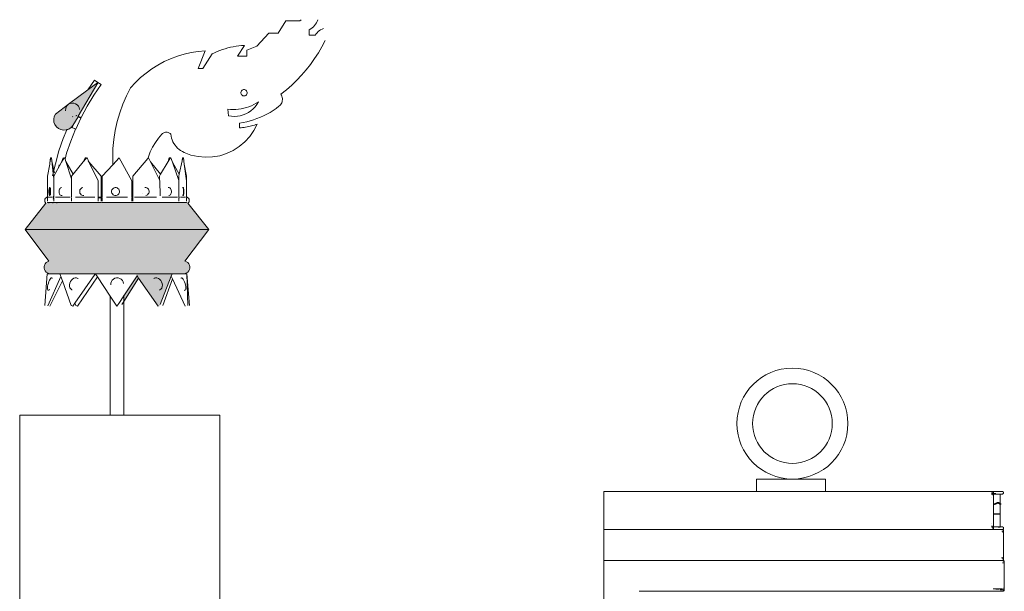
# Model space of a CAD drawing. Units: millimetres. Extents: x 2322 to 2394, y 1600 to 1790.
# Tile 5 of 5: x 2322 to 2380, y 1757 to 1790. Entities that reach past the tile are written whole.
import ezdxf

# ---------------------------------------------------------------- set-up
doc = ezdxf.new("R2010")
doc.units = ezdxf.units.MM
doc.layers.add('A-FURN-ACCS', color=8, linetype='Continuous', lineweight=18)
doc.layers.add('A-FURN-PATT', color=18, linetype='Continuous', lineweight=13)

msp = doc.modelspace()

# ---------------------------------------------------------------- hatches: boundary and pattern name
at = {"layer": 'A-FURN-PATT'}
h = msp.add_hatch(color=256, dxfattribs=at)
h.dxf.hatch_style = 1
h.paths.add_polyline_path([(2326.67, 1786.535), (2326.67, 1786.566), (2326.085, 1786.128), (2324.955, 1785.277), (2324.18, 1784.703), (2324.111, 1784.565), (2324.082, 1784.414), (2324.082, 1784.383), (2324.093, 1784.23), (2324.146, 1784.085), (2324.235, 1783.958), (2324.355, 1783.858), (2324.499, 1783.791), (2324.655, 1783.762), (2324.813, 1783.774), (2324.846, 1783.785), (2324.963, 1783.824), (2325.095, 1783.911), (2325.116, 1783.935), (2325.199, 1784.027), (2325.505, 1784.55), (2325.522, 1784.578)])
h = msp.add_hatch(color=256, dxfattribs=at)
h.dxf.hatch_style = 1
h.paths.add_polyline_path([(2331.932, 1779.508), (2331.431, 1779.508), (2328.723, 1779.508), (2328.671, 1779.508), (2326.915, 1779.508), (2326.693, 1779.508), (2325.129, 1779.508), (2324.26, 1779.508), (2324.078, 1779.508), (2323.654, 1779.508), (2322.407, 1777.93), (2333.179, 1777.93)])
h.paths.add_polyline_path([(2329.065, 1775.075), (2328.192, 1773.709), (2328.192, 1774.037), (2328.972, 1775.209), (2328.887, 1775.333), (2328.806, 1775.334), (2326.559, 1775.334), (2326.559, 1775.291), (2326.583, 1775.254), (2326.403, 1775.334), (2324.439, 1775.334), (2324.444, 1775.321), (2324.403, 1775.334), (2323.879, 1775.334), (2323.714, 1775.334), (2323.509, 1775.569), (2323.513, 1775.85), (2323.761, 1776.118), (2322.407, 1777.93), (2333.179, 1777.93), (2331.799, 1776.084), (2332.026, 1775.934), (2332.098, 1775.662), (2331.897, 1775.269), (2331.896, 1775.318), (2331.894, 1775.332), (2331.707, 1775.334), (2331.079, 1775.334), (2331.03, 1775.32), (2330.978, 1775.187), (2330.253, 1773.35)])
h.paths.add_polyline_path([(2330.421, 1774.493), (2330.451, 1774.574), (2330.46, 1774.664), (2330.448, 1774.759), (2330.415, 1774.851), (2330.364, 1774.935), (2330.298, 1775.004), (2330.222, 1775.053), (2330.104, 1775.093), (2330.07, 1775.083), (2330.227, 1775.078), (2330.435, 1774.861), (2330.473, 1774.563)], flags=16)

# ---------------------------------------------------------------- linework, layer by layer
at = {"layer": 'A-FURN-ACCS'}
for p, q in [((2337.261, 1789.455), (2337.707, 1790.174)), ((2337.707, 1790.174), (2338.529, 1790.174)), ((2338.529, 1790.174), (2338.606, 1790.244)), ((2339.456, 1789.973), (2339.394, 1789.895)), ((2339.51, 1790.056), (2339.456, 1789.973)), ((2339.556, 1790.144), (2339.51, 1790.056)), ((2339.593, 1790.236), (2339.556, 1790.144)), ((2336.01, 1788.693), (2336.709, 1789.455)), ((2336.709, 1789.455), (2337.261, 1789.455)), ((2339.17, 1789.701), (2339.084, 1789.652)), ((2339.084, 1789.652), (2339.084, 1789.334)), ((2339.251, 1789.758), (2339.17, 1789.701)), ((2339.326, 1789.823), (2339.251, 1789.758)), ((2339.394, 1789.895), (2339.326, 1789.823)), ((2339.436, 1789.334), (2339.487, 1789.409)), ((2339.487, 1789.409), (2339.544, 1789.479)), ((2339.544, 1789.479), (2339.608, 1789.542)), ((2339.608, 1789.542), (2339.677, 1789.6)), ((2339.677, 1789.6), (2339.752, 1789.65)), ((2339.752, 1789.65), (2339.832, 1789.693)), ((2339.832, 1789.693), (2339.915, 1789.727)), ((2339.084, 1789.334), (2339.436, 1789.334)), ((2340.022, 1789.023), (2339.828, 1788.659)), ((2331.738, 1788.218), (2332.147, 1788.31)), ((2332.147, 1788.31), (2332.561, 1788.373)), ((2332.561, 1788.373), (2332.978, 1788.408)), ((2332.978, 1788.408), (2332.568, 1787.37)), ((2332.827, 1787.37), (2333.378, 1788.231)), ((2333.378, 1788.231), (2333.526, 1788.304)), ((2333.526, 1788.304), (2333.677, 1788.371)), ((2333.677, 1788.371), (2333.829, 1788.433)), ((2333.829, 1788.433), (2333.984, 1788.489)), ((2333.984, 1788.489), (2334.141, 1788.54)), ((2334.141, 1788.54), (2334.299, 1788.585)), ((2334.299, 1788.585), (2334.459, 1788.624)), ((2334.459, 1788.624), (2334.621, 1788.658)), ((2334.621, 1788.658), (2334.783, 1788.686)), ((2334.783, 1788.686), (2334.946, 1788.708)), ((2335.275, 1788.734), (2334.869, 1788.101)), ((2334.946, 1788.708), (2335.11, 1788.724)), ((2335.11, 1788.724), (2335.275, 1788.734)), ((2335.41, 1788.454), (2336.01, 1788.693)), ((2335.41, 1788.101), (2335.41, 1788.454)), ((2339.619, 1788.304), (2339.394, 1787.958)), ((2339.828, 1788.659), (2339.619, 1788.304)), ((2330.193, 1787.583), (2330.562, 1787.78)), ((2330.562, 1787.78), (2330.944, 1787.953)), ((2330.944, 1787.953), (2331.337, 1788.099)), ((2331.337, 1788.099), (2331.738, 1788.218)), ((2334.869, 1788.101), (2335.41, 1788.101)), ((2339.394, 1787.958), (2339.154, 1787.623)), ((2329.178, 1786.845), (2329.5, 1787.114)), ((2329.5, 1787.114), (2329.839, 1787.36)), ((2329.839, 1787.36), (2330.193, 1787.583)), ((2332.568, 1787.37), (2332.827, 1787.37)), ((2338.899, 1787.299), (2338.63, 1786.987)), ((2339.154, 1787.623), (2338.899, 1787.299)), ((2326.67, 1786.535), (2325.522, 1784.578)), ((2326.476, 1786.699), (2326.085, 1786.128)), ((2326.67, 1786.566), (2326.085, 1786.128)), ((2326.67, 1786.566), (2326.476, 1786.699)), ((2326.67, 1786.535), (2326.67, 1786.566)), ((2326.864, 1786.433), (2326.67, 1786.566)), ((2328.594, 1786.246), (2328.876, 1786.556)), ((2328.876, 1786.556), (2329.178, 1786.845)), ((2338.347, 1786.687), (2338.051, 1786.4)), ((2338.63, 1786.987), (2338.347, 1786.687)), ((2326.085, 1786.128), (2324.955, 1785.277)), ((2326.434, 1785.805), (2326.864, 1786.433)), ((2328.594, 1786.246), (2328.353, 1785.77)), ((2335.066, 1785.929), (2335.067, 1785.979)), ((2335.079, 1785.882), (2335.066, 1785.929)), ((2335.067, 1785.979), (2335.08, 1786.026)), ((2335.08, 1786.026), (2335.104, 1786.068)), ((2335.104, 1786.068), (2335.139, 1786.103)), ((2335.139, 1786.103), (2335.182, 1786.127)), ((2335.182, 1786.127), (2335.229, 1786.14)), ((2335.229, 1786.14), (2335.278, 1786.139)), ((2335.278, 1786.139), (2335.326, 1786.126)), ((2335.326, 1786.126), (2335.368, 1786.102)), ((2335.368, 1786.102), (2335.403, 1786.067)), ((2335.403, 1786.067), (2335.427, 1786.024)), ((2335.439, 1785.928), (2335.426, 1785.88)), ((2335.427, 1786.024), (2335.439, 1785.977)), ((2335.439, 1785.977), (2335.439, 1785.928)), ((2337.743, 1786.126), (2337.422, 1785.867)), ((2338.051, 1786.4), (2337.743, 1786.126)), ((2325.051, 1785.324), (2325.156, 1785.346)), ((2325.156, 1785.346), (2325.263, 1785.341)), ((2325.263, 1785.341), (2325.365, 1785.308)), ((2326.042, 1785.161), (2326.434, 1785.805)), ((2328.353, 1785.77), (2328.142, 1785.279)), ((2335.103, 1785.839), (2335.079, 1785.882)), ((2335.138, 1785.804), (2335.103, 1785.839)), ((2335.18, 1785.78), (2335.138, 1785.804)), ((2335.227, 1785.767), (2335.18, 1785.78)), ((2335.276, 1785.767), (2335.227, 1785.767)), ((2335.324, 1785.779), (2335.276, 1785.767)), ((2335.367, 1785.803), (2335.324, 1785.779)), ((2335.401, 1785.838), (2335.367, 1785.803)), ((2335.426, 1785.88), (2335.401, 1785.838)), ((2335.966, 1785.337), (2335.828, 1785.261)), ((2336.099, 1785.421), (2335.966, 1785.337)), ((2336.099, 1785.421), (2336.008, 1785.273)), ((2337.422, 1785.867), (2337.455, 1785.81)), ((2337.465, 1785.364), (2337.435, 1785.306)), ((2337.455, 1785.81), (2337.48, 1785.749)), ((2337.488, 1785.426), (2337.465, 1785.364)), ((2337.48, 1785.749), (2337.498, 1785.686)), ((2337.502, 1785.49), (2337.488, 1785.426)), ((2337.498, 1785.686), (2337.508, 1785.621)), ((2337.509, 1785.555), (2337.502, 1785.49)), ((2337.508, 1785.621), (2337.509, 1785.555)), ((2324.955, 1785.277), (2324.18, 1784.703)), ((2324.778, 1784.919), (2324.784, 1785.022)), ((2324.779, 1784.915), (2324.778, 1784.919)), ((2324.778, 1784.901), (2324.779, 1784.915)), ((2324.784, 1785.022), (2324.817, 1785.121)), ((2324.817, 1785.121), (2324.875, 1785.208)), ((2324.875, 1785.208), (2324.955, 1785.277)), ((2324.955, 1785.277), (2325.051, 1785.324)), ((2325.365, 1785.308), (2325.455, 1785.252)), ((2325.455, 1785.252), (2325.527, 1785.175)), ((2325.527, 1785.175), (2325.576, 1785.082)), ((2325.576, 1785.082), (2325.598, 1784.981)), ((2325.597, 1784.966), (2325.598, 1784.981)), ((2325.597, 1784.966), (2325.598, 1784.963)), ((2326.042, 1785.161), (2325.685, 1784.496)), ((2327.961, 1784.776), (2327.812, 1784.264)), ((2328.142, 1785.279), (2327.961, 1784.776)), ((2334.462, 1784.972), (2334.306, 1784.985)), ((2334.306, 1784.985), (2334.344, 1784.595)), ((2334.619, 1784.968), (2334.462, 1784.972)), ((2334.776, 1784.973), (2334.619, 1784.968)), ((2334.932, 1784.987), (2334.776, 1784.973)), ((2335.087, 1785.011), (2334.932, 1784.987)), ((2335.241, 1785.043), (2335.087, 1785.011)), ((2335.392, 1785.085), (2335.241, 1785.043)), ((2335.509, 1784.802), (2335.357, 1784.721)), ((2335.541, 1785.135), (2335.392, 1785.085)), ((2335.652, 1784.9), (2335.509, 1784.802)), ((2335.687, 1785.194), (2335.541, 1785.135)), ((2335.783, 1785.012), (2335.652, 1784.9)), ((2335.828, 1785.261), (2335.687, 1785.194)), ((2335.903, 1785.137), (2335.783, 1785.012)), ((2336.008, 1785.273), (2335.903, 1785.137)), ((2336.778, 1784.805), (2336.593, 1784.702)), ((2336.958, 1784.916), (2336.778, 1784.805)), ((2337.134, 1785.034), (2336.958, 1784.916)), ((2337.304, 1785.16), (2337.134, 1785.034)), ((2337.354, 1785.203), (2337.304, 1785.16)), ((2337.397, 1785.252), (2337.354, 1785.203)), ((2337.435, 1785.306), (2337.397, 1785.252)), ((2324.111, 1784.565), (2324.082, 1784.414)), ((2324.082, 1784.383), (2324.082, 1784.414)), ((2324.082, 1784.383), (2324.093, 1784.23)), ((2324.093, 1784.23), (2324.146, 1784.085)), ((2324.18, 1784.703), (2324.111, 1784.565)), ((2325.194, 1784.555), (2325.185, 1784.537)), ((2325.505, 1784.55), (2325.199, 1784.027)), ((2325.367, 1783.817), (2325.673, 1784.471)), ((2325.386, 1784.605), (2325.405, 1784.597)), ((2325.438, 1784.619), (2325.425, 1784.626)), ((2325.522, 1784.578), (2325.505, 1784.55)), ((2325.673, 1784.471), (2325.505, 1784.55)), ((2325.522, 1784.578), (2325.685, 1784.496)), ((2327.812, 1784.264), (2327.695, 1783.743)), ((2334.515, 1784.571), (2334.344, 1784.595)), ((2334.688, 1784.565), (2334.515, 1784.571)), ((2334.86, 1784.577), (2334.688, 1784.565)), ((2335.031, 1784.607), (2334.86, 1784.577)), ((2335.201, 1784.208), (2334.992, 1784.171)), ((2335.197, 1784.656), (2335.031, 1784.607)), ((2335.357, 1784.721), (2335.197, 1784.656)), ((2335.408, 1784.253), (2335.201, 1784.208)), ((2335.612, 1784.307), (2335.408, 1784.253)), ((2335.815, 1784.369), (2335.612, 1784.307)), ((2336.014, 1784.44), (2335.815, 1784.369)), ((2336.211, 1784.519), (2336.014, 1784.44)), ((2336.404, 1784.606), (2336.211, 1784.519)), ((2336.593, 1784.702), (2336.404, 1784.606)), ((2324.146, 1784.085), (2324.235, 1783.958)), ((2324.235, 1783.958), (2324.355, 1783.858)), ((2324.355, 1783.858), (2324.499, 1783.791)), ((2324.499, 1783.791), (2324.655, 1783.762)), ((2324.846, 1783.785), (2324.641, 1783.277)), ((2324.655, 1783.762), (2324.813, 1783.774)), ((2324.813, 1783.774), (2324.846, 1783.785)), ((2324.846, 1783.785), (2324.963, 1783.824)), ((2324.861, 1783.82), (2324.846, 1783.785)), ((2324.963, 1783.824), (2325.095, 1783.911)), ((2325.082, 1783.113), (2325.364, 1783.812)), ((2325.085, 1783.934), (2325.107, 1783.925)), ((2325.095, 1783.911), (2325.107, 1783.925)), ((2325.116, 1783.935), (2325.099, 1783.943)), ((2325.107, 1783.925), (2325.116, 1783.935)), ((2325.107, 1783.925), (2325.364, 1783.812)), ((2325.116, 1783.935), (2325.199, 1784.027)), ((2325.116, 1783.935), (2325.367, 1783.817)), ((2325.154, 1783.917), (2325.149, 1783.906)), ((2325.232, 1784.084), (2325.154, 1783.917)), ((2327.695, 1783.743), (2327.611, 1783.215)), ((2330.546, 1783.61), (2330.502, 1783.587)), ((2330.593, 1783.627), (2330.546, 1783.61)), ((2330.641, 1783.637), (2330.593, 1783.627)), ((2330.691, 1783.641), (2330.641, 1783.637)), ((2330.74, 1783.637), (2330.691, 1783.641)), ((2330.789, 1783.627), (2330.74, 1783.637)), ((2330.835, 1783.61), (2330.789, 1783.627)), ((2330.879, 1783.587), (2330.835, 1783.61)), ((2334.992, 1784.171), (2334.992, 1783.901)), ((2334.992, 1783.901), (2335.081, 1783.905)), ((2335.081, 1783.905), (2335.169, 1783.912)), ((2335.169, 1783.912), (2335.257, 1783.921)), ((2335.257, 1783.921), (2335.345, 1783.933)), ((2335.345, 1783.933), (2335.432, 1783.948)), ((2335.432, 1783.948), (2335.519, 1783.965)), ((2335.519, 1783.965), (2335.605, 1783.984)), ((2335.832, 1783.74), (2335.589, 1783.389)), ((2335.605, 1783.984), (2335.691, 1784.007)), ((2335.691, 1784.007), (2335.776, 1784.031)), ((2335.776, 1784.031), (2335.861, 1784.059)), ((2336.027, 1784.12), (2335.832, 1783.74)), ((2335.861, 1784.059), (2335.944, 1784.088)), ((2335.944, 1784.088), (2336.027, 1784.12)), ((2324.641, 1783.277), (2324.388, 1782.539)), ((2324.837, 1782.399), (2325.082, 1783.113)), ((2327.611, 1783.215), (2327.559, 1782.684)), ((2330.048, 1783.031), (2329.888, 1782.763)), ((2330.227, 1783.284), (2330.048, 1783.031)), ((2330.426, 1783.523), (2330.227, 1783.284)), ((2330.462, 1783.558), (2330.426, 1783.523)), ((2330.502, 1783.587), (2330.462, 1783.558)), ((2330.919, 1783.558), (2330.879, 1783.587)), ((2330.955, 1783.523), (2330.919, 1783.558)), ((2330.972, 1783.409), (2330.955, 1783.523)), ((2330.999, 1783.296), (2330.972, 1783.409)), ((2331.036, 1783.186), (2330.999, 1783.296)), ((2331.082, 1783.08), (2331.036, 1783.186)), ((2331.137, 1782.978), (2331.082, 1783.08)), ((2335.303, 1783.073), (2334.976, 1782.798)), ((2335.589, 1783.389), (2335.303, 1783.073)), ((2324.388, 1782.539), (2324.175, 1781.789)), ((2327.559, 1782.684), (2327.54, 1782.15)), ((2329.751, 1782.484), (2329.636, 1782.195)), ((2329.888, 1782.763), (2329.751, 1782.484)), ((2331.201, 1782.882), (2331.137, 1782.978)), ((2331.273, 1782.791), (2331.201, 1782.882)), ((2331.353, 1782.707), (2331.273, 1782.791)), ((2331.439, 1782.63), (2331.353, 1782.707)), ((2331.532, 1782.561), (2331.439, 1782.63)), ((2331.631, 1782.5), (2331.532, 1782.561)), ((2331.734, 1782.448), (2331.631, 1782.5)), ((2332.135, 1782.3), (2331.734, 1782.448)), ((2334.617, 1782.567), (2334.23, 1782.386)), ((2334.976, 1782.798), (2334.617, 1782.567)), ((2323.85, 1781.835), (2323.888, 1782.128)), ((2323.907, 1782.128), (2323.85, 1781.835)), ((2323.907, 1782.128), (2323.888, 1782.128)), ((2323.907, 1782.128), (2323.953, 1782.128)), ((2323.97, 1781.96), (2323.953, 1782.128)), ((2323.97, 1781.96), (2324.09, 1781.413)), ((2324.047, 1781.22), (2323.97, 1781.96)), ((2324.539, 1781.875), (2324.078, 1781.061)), ((2324.539, 1781.875), (2324.627, 1782.128)), ((2324.683, 1782.128), (2324.539, 1781.875)), ((2324.638, 1782.128), (2324.627, 1782.128)), ((2324.72, 1782.128), (2324.683, 1782.128)), ((2324.742, 1782.063), (2324.72, 1782.128)), ((2324.742, 1782.063), (2324.837, 1782.399)), ((2324.789, 1781.918), (2324.742, 1782.063)), ((2324.789, 1781.918), (2325.229, 1781.185)), ((2325.126, 1780.892), (2324.789, 1781.918)), ((2325.817, 1781.891), (2325.229, 1781.185)), ((2325.817, 1781.891), (2325.934, 1782.128)), ((2325.985, 1782.093), (2325.817, 1781.891)), ((2325.955, 1782.128), (2325.934, 1782.128)), ((2325.955, 1782.128), (2325.985, 1782.093)), ((2326.015, 1782.128), (2325.985, 1782.093)), ((2326.037, 1782.128), (2326.015, 1782.128)), ((2326.144, 1781.905), (2326.037, 1782.128)), ((2326.093, 1781.966), (2326.144, 1781.905)), ((2326.144, 1781.905), (2326.863, 1781.061)), ((2326.683, 1780.789), (2326.144, 1781.905)), ((2327.54, 1782.15), (2327.551, 1781.733)), ((2327.925, 1782.128), (2327.551, 1781.733)), ((2328.66, 1780.789), (2327.925, 1782.128)), ((2329.603, 1782.09), (2328.723, 1781.061)), ((2329.603, 1782.09), (2329.594, 1782.061)), ((2329.606, 1782.099), (2329.603, 1782.09)), ((2329.603, 1782.09), (2329.611, 1782.08)), ((2329.636, 1782.195), (2329.606, 1782.099)), ((2329.631, 1782.128), (2329.606, 1782.099)), ((2329.631, 1782.128), (2329.652, 1782.128)), ((2329.768, 1781.891), (2329.652, 1782.128)), ((2329.768, 1781.891), (2330.357, 1781.185)), ((2329.768, 1781.891), (2330.283, 1780.849)), ((2330.797, 1781.918), (2330.357, 1781.185)), ((2330.797, 1781.918), (2330.866, 1782.128)), ((2330.913, 1782.112), (2330.797, 1781.918)), ((2330.866, 1782.128), (2330.903, 1782.128)), ((2330.903, 1782.128), (2330.913, 1782.112)), ((2330.923, 1782.128), (2330.913, 1782.112)), ((2330.923, 1782.128), (2330.959, 1782.128)), ((2331.047, 1781.875), (2330.959, 1782.128)), ((2331.047, 1781.875), (2331.444, 1781.175)), ((2331.047, 1781.875), (2331.419, 1780.805)), ((2331.616, 1781.96), (2331.444, 1781.175)), ((2331.616, 1781.96), (2331.633, 1782.128)), ((2331.653, 1782.128), (2331.616, 1781.96)), ((2331.633, 1782.128), (2331.653, 1782.128)), ((2331.653, 1782.128), (2331.698, 1782.128)), ((2331.698, 1782.128), (2331.745, 1781.762)), ((2332.551, 1782.205), (2332.135, 1782.3)), ((2332.976, 1782.167), (2332.551, 1782.205)), ((2333.403, 1782.184), (2332.976, 1782.167)), ((2333.823, 1782.258), (2333.403, 1782.184)), ((2334.23, 1782.386), (2333.823, 1782.258)), ((2323.841, 1781.762), (2323.716, 1781.061)), ((2323.841, 1781.762), (2323.85, 1781.835)), ((2324.09, 1781.413), (2324.047, 1781.22)), ((2324.175, 1781.789), (2324.09, 1781.413)), ((2324.09, 1781.413), (2324.125, 1781.254)), ((2324.403, 1781.731), (2324.367, 1781.572)), ((2327.551, 1781.733), (2326.915, 1781.061)), ((2331.745, 1781.762), (2331.87, 1781.061)), ((2331.869, 1780.789), (2331.745, 1781.762)), ((2323.717, 1780.789), (2323.715, 1779.832)), ((2323.716, 1781.061), (2323.719, 1780.805)), ((2323.717, 1780.789), (2323.719, 1780.805)), ((2324.047, 1781.22), (2324.015, 1781.08)), ((2324.078, 1780.924), (2324.047, 1781.22)), ((2324.078, 1781.061), (2324.078, 1780.924)), ((2324.078, 1780.924), (2324.078, 1779.835)), ((2325.229, 1781.185), (2325.126, 1781.061)), ((2325.126, 1781.061), (2325.126, 1780.892)), ((2325.126, 1780.892), (2325.126, 1779.822)), ((2326.683, 1780.789), (2326.69, 1779.835)), ((2326.863, 1781.061), (2326.863, 1779.835)), ((2326.915, 1781.061), (2326.915, 1779.835)), ((2328.66, 1780.789), (2328.666, 1780.042)), ((2328.723, 1781.061), (2328.723, 1780.042)), ((2330.357, 1781.185), (2330.283, 1781.061)), ((2330.283, 1781.061), (2330.283, 1780.849)), ((2330.312, 1780.789), (2330.283, 1780.849)), ((2330.312, 1780.789), (2330.319, 1779.907)), ((2331.444, 1781.175), (2331.419, 1781.061)), ((2331.419, 1781.061), (2331.419, 1780.805)), ((2331.424, 1780.789), (2331.419, 1780.805)), ((2331.424, 1780.789), (2331.429, 1779.835)), ((2331.87, 1781.061), (2331.869, 1780.789)), ((2331.869, 1780.789), (2331.87, 1779.832)), ((2323.798, 1780.188), (2323.801, 1780.247)), ((2323.798, 1780.127), (2323.798, 1780.188)), ((2323.801, 1780.247), (2323.807, 1780.3)), ((2323.807, 1780.3), (2323.815, 1780.344)), ((2323.815, 1780.344), (2323.825, 1780.374)), ((2323.821, 1780.188), (2323.824, 1780.247)), ((2323.821, 1780.127), (2323.821, 1780.188)), ((2323.824, 1780.247), (2323.83, 1780.3)), ((2323.825, 1780.374), (2323.837, 1780.39)), ((2323.83, 1780.3), (2323.838, 1780.344)), ((2323.86, 1780.39), (2323.837, 1780.39)), ((2323.838, 1780.344), (2323.848, 1780.374)), ((2323.848, 1780.374), (2323.86, 1780.39)), ((2323.865, 1780.246), (2323.861, 1780.187)), ((2323.861, 1780.187), (2323.861, 1780.126)), ((2323.872, 1780.299), (2323.865, 1780.246)), ((2323.873, 1780.259), (2323.865, 1780.246)), ((2323.882, 1780.343), (2323.872, 1780.299)), ((2323.872, 1780.299), (2323.873, 1780.259)), ((2323.888, 1780.357), (2323.882, 1780.343)), ((2323.889, 1780.354), (2323.882, 1780.343)), ((2323.888, 1780.246), (2323.884, 1780.187)), ((2323.884, 1780.187), (2323.884, 1780.126)), ((2323.895, 1780.299), (2323.888, 1780.246)), ((2323.898, 1780.313), (2323.895, 1780.299)), ((2324.394, 1780.188), (2324.403, 1780.247)), ((2324.394, 1780.127), (2324.394, 1780.188)), ((2324.403, 1780.247), (2324.422, 1780.3)), ((2324.422, 1780.3), (2324.448, 1780.344)), ((2324.448, 1780.344), (2324.48, 1780.374)), ((2324.48, 1780.374), (2324.515, 1780.39)), ((2324.534, 1780.39), (2324.515, 1780.39)), ((2325.607, 1780.188), (2325.621, 1780.247)), ((2325.607, 1780.127), (2325.607, 1780.188)), ((2325.621, 1780.247), (2325.648, 1780.3)), ((2325.648, 1780.3), (2325.686, 1780.344)), ((2325.686, 1780.344), (2325.733, 1780.374)), ((2325.733, 1780.374), (2325.785, 1780.39)), ((2325.796, 1780.39), (2325.785, 1780.39)), ((2327.474, 1780.188), (2327.49, 1780.247)), ((2327.474, 1780.127), (2327.474, 1780.188)), ((2327.49, 1780.247), (2327.521, 1780.3)), ((2327.521, 1780.3), (2327.564, 1780.344)), ((2327.564, 1780.344), (2327.618, 1780.374)), ((2327.618, 1780.374), (2327.677, 1780.39)), ((2327.677, 1780.39), (2327.738, 1780.39)), ((2327.738, 1780.39), (2327.798, 1780.374)), ((2327.798, 1780.374), (2327.851, 1780.343)), ((2327.851, 1780.343), (2327.894, 1780.299)), ((2327.894, 1780.299), (2327.924, 1780.246)), ((2327.924, 1780.246), (2327.94, 1780.187)), ((2327.94, 1780.187), (2327.94, 1780.126)), ((2329.428, 1780.39), (2329.439, 1780.39)), ((2329.439, 1780.39), (2329.494, 1780.39)), ((2329.494, 1780.39), (2329.547, 1780.374)), ((2329.547, 1780.374), (2329.595, 1780.343)), ((2329.595, 1780.343), (2329.634, 1780.299)), ((2329.634, 1780.299), (2329.661, 1780.246)), ((2329.661, 1780.246), (2329.675, 1780.187)), ((2329.675, 1780.187), (2329.675, 1780.126)), ((2330.802, 1780.39), (2330.82, 1780.39)), ((2330.82, 1780.39), (2330.859, 1780.39)), ((2330.859, 1780.39), (2330.896, 1780.374)), ((2330.896, 1780.374), (2330.93, 1780.343)), ((2330.93, 1780.343), (2330.957, 1780.299)), ((2330.957, 1780.299), (2330.977, 1780.246)), ((2330.977, 1780.246), (2330.987, 1780.187)), ((2330.987, 1780.187), (2330.987, 1780.126)), ((2331.641, 1780.39), (2331.655, 1780.39)), ((2331.655, 1780.39), (2331.669, 1780.374)), ((2331.655, 1780.39), (2331.664, 1780.39)), ((2331.664, 1780.39), (2331.678, 1780.39)), ((2331.669, 1780.374), (2331.681, 1780.343)), ((2331.678, 1780.39), (2331.692, 1780.374)), ((2331.681, 1780.343), (2331.691, 1780.299)), ((2331.691, 1780.299), (2331.698, 1780.246)), ((2331.692, 1780.374), (2331.704, 1780.343)), ((2331.698, 1780.246), (2331.702, 1780.187)), ((2331.702, 1780.187), (2331.702, 1780.126)), ((2331.704, 1780.343), (2331.714, 1780.299)), ((2331.714, 1780.299), (2331.721, 1780.246)), ((2331.721, 1780.246), (2331.725, 1780.187)), ((2331.725, 1780.187), (2331.725, 1780.126)), ((2323.547, 1779.607), (2323.548, 1779.66)), ((2323.56, 1779.555), (2323.547, 1779.607)), ((2323.548, 1779.66), (2323.563, 1779.712)), ((2323.587, 1779.508), (2323.56, 1779.555)), ((2323.563, 1779.712), (2323.59, 1779.758)), ((2323.59, 1779.758), (2323.629, 1779.796)), ((2323.629, 1779.796), (2323.675, 1779.822)), ((2323.675, 1779.822), (2323.715, 1779.832)), ((2323.715, 1779.832), (2323.728, 1779.835)), ((2323.715, 1779.832), (2323.715, 1779.822)), ((2323.715, 1779.796), (2323.715, 1779.607)), ((2323.715, 1779.555), (2323.715, 1779.508)), ((2323.728, 1779.835), (2323.737, 1779.835)), ((2323.728, 1779.835), (2323.731, 1779.835)), ((2324.003, 1779.835), (2323.737, 1779.835)), ((2323.801, 1780.067), (2323.798, 1780.127)), ((2323.807, 1780.014), (2323.801, 1780.067)), ((2323.815, 1779.971), (2323.807, 1780.014)), ((2323.825, 1779.94), (2323.815, 1779.971)), ((2323.824, 1780.067), (2323.821, 1780.127)), ((2323.83, 1780.014), (2323.824, 1780.067)), ((2323.836, 1779.924), (2323.825, 1779.94)), ((2323.838, 1779.971), (2323.83, 1780.014)), ((2323.848, 1779.924), (2323.836, 1779.924)), ((2323.861, 1780.126), (2323.838, 1779.971)), ((2323.848, 1779.94), (2323.838, 1779.971)), ((2323.859, 1779.924), (2323.848, 1779.94)), ((2323.859, 1779.924), (2323.848, 1779.924)), ((2323.871, 1779.924), (2323.859, 1779.924)), ((2323.861, 1780.126), (2323.865, 1780.066)), ((2323.865, 1780.066), (2323.872, 1780.013)), ((2323.872, 1780.013), (2323.882, 1779.97)), ((2323.882, 1779.97), (2323.888, 1779.956)), ((2323.884, 1780.126), (2323.888, 1780.066)), ((2323.888, 1780.066), (2323.895, 1780.013)), ((2323.895, 1780.013), (2323.898, 1780)), ((2324.078, 1779.835), (2324.047, 1779.835)), ((2324.056, 1779.796), (2324.047, 1779.715)), ((2324.078, 1779.792), (2324.047, 1779.792)), ((2324.078, 1779.981), (2324.059, 1779.822)), ((2324.078, 1779.835), (2324.078, 1779.822)), ((2324.078, 1779.796), (2324.078, 1779.792)), ((2324.078, 1779.792), (2324.078, 1779.607)), ((2324.078, 1779.555), (2324.078, 1779.508)), ((2325.038, 1779.835), (2324.189, 1779.835)), ((2324.403, 1780.067), (2324.394, 1780.127)), ((2324.421, 1780.014), (2324.403, 1780.067)), ((2324.447, 1779.971), (2324.421, 1780.014)), ((2324.479, 1779.94), (2324.447, 1779.971)), ((2324.514, 1779.924), (2324.479, 1779.94)), ((2324.551, 1779.924), (2324.514, 1779.924)), ((2324.57, 1779.924), (2324.551, 1779.924)), ((2325.126, 1779.796), (2325.126, 1779.607)), ((2325.126, 1779.555), (2325.129, 1779.508)), ((2325.355, 1779.835), (2326.485, 1779.835)), ((2325.62, 1780.067), (2325.607, 1780.127)), ((2325.647, 1780.014), (2325.62, 1780.067)), ((2325.685, 1779.971), (2325.647, 1780.014)), ((2325.732, 1779.94), (2325.685, 1779.971)), ((2325.784, 1779.924), (2325.732, 1779.94)), ((2325.838, 1779.924), (2325.784, 1779.924)), ((2325.849, 1779.924), (2325.838, 1779.924)), ((2326.69, 1779.835), (2326.668, 1779.835)), ((2326.691, 1779.792), (2326.668, 1779.792)), ((2326.69, 1779.835), (2326.691, 1779.822)), ((2326.863, 1779.835), (2326.69, 1779.835)), ((2326.691, 1779.796), (2326.691, 1779.792)), ((2326.691, 1779.792), (2326.692, 1779.607)), ((2326.863, 1779.792), (2326.691, 1779.792)), ((2326.693, 1779.555), (2326.693, 1779.508)), ((2326.863, 1779.835), (2326.915, 1779.835)), ((2326.863, 1779.835), (2326.863, 1779.822)), ((2326.863, 1779.796), (2326.863, 1779.792)), ((2326.863, 1779.792), (2326.863, 1779.607)), ((2326.915, 1779.792), (2326.863, 1779.792)), ((2326.863, 1779.555), (2326.863, 1779.508)), ((2326.915, 1779.835), (2326.915, 1779.822)), ((2326.915, 1779.796), (2326.915, 1779.792)), ((2326.915, 1779.792), (2326.915, 1779.607)), ((2326.915, 1779.555), (2326.915, 1779.508)), ((2327.168, 1779.835), (2328.418, 1779.835)), ((2327.49, 1780.067), (2327.474, 1780.127)), ((2327.52, 1780.014), (2327.49, 1780.067)), ((2327.563, 1779.971), (2327.52, 1780.014)), ((2327.617, 1779.94), (2327.563, 1779.971)), ((2327.676, 1779.924), (2327.617, 1779.94)), ((2327.737, 1779.924), (2327.676, 1779.924)), ((2327.796, 1779.939), (2327.737, 1779.924)), ((2327.85, 1779.97), (2327.796, 1779.939)), ((2327.893, 1780.013), (2327.85, 1779.97)), ((2327.924, 1780.066), (2327.893, 1780.013)), ((2327.94, 1780.126), (2327.924, 1780.066)), ((2328.723, 1780.042), (2328.666, 1780.042)), ((2328.666, 1780.042), (2328.668, 1779.835)), ((2328.668, 1779.835), (2328.668, 1779.822)), ((2328.723, 1779.835), (2328.668, 1779.835)), ((2328.668, 1779.796), (2328.668, 1779.792)), ((2328.668, 1779.792), (2328.67, 1779.607)), ((2328.723, 1779.792), (2328.668, 1779.792)), ((2328.67, 1779.555), (2328.671, 1779.508)), ((2328.743, 1780.042), (2328.723, 1780.042)), ((2328.723, 1780.042), (2328.723, 1779.835)), ((2328.743, 1779.835), (2328.723, 1779.835)), ((2328.723, 1779.835), (2328.723, 1779.822)), ((2328.723, 1779.796), (2328.723, 1779.792)), ((2328.743, 1779.792), (2328.723, 1779.792)), ((2328.723, 1779.792), (2328.723, 1779.607)), ((2328.723, 1779.555), (2328.723, 1779.508)), ((2328.817, 1779.835), (2330.109, 1779.835)), ((2329.281, 1780.047), (2329.271, 1780.047)), ((2329.483, 1779.924), (2329.493, 1779.924)), ((2329.546, 1779.939), (2329.493, 1779.924)), ((2329.594, 1779.97), (2329.546, 1779.939)), ((2329.633, 1780.013), (2329.594, 1779.97)), ((2329.661, 1780.066), (2329.633, 1780.013)), ((2329.675, 1780.126), (2329.661, 1780.066)), ((2331.352, 1779.835), (2330.452, 1779.835)), ((2330.84, 1779.924), (2330.858, 1779.924)), ((2330.896, 1779.939), (2330.858, 1779.924)), ((2330.929, 1779.97), (2330.896, 1779.939)), ((2330.957, 1780.013), (2330.929, 1779.97)), ((2330.976, 1780.066), (2330.957, 1780.013)), ((2330.987, 1780.126), (2330.976, 1780.066)), ((2331.464, 1779.835), (2331.429, 1779.835)), ((2331.429, 1779.835), (2331.43, 1779.822)), ((2331.43, 1779.796), (2331.43, 1779.792)), ((2331.464, 1779.792), (2331.43, 1779.792)), ((2331.43, 1779.792), (2331.431, 1779.607)), ((2331.431, 1779.555), (2331.431, 1779.508)), ((2331.525, 1779.835), (2331.822, 1779.835)), ((2331.668, 1779.939), (2331.655, 1779.924)), ((2331.655, 1779.924), (2331.678, 1779.924)), ((2331.681, 1779.97), (2331.668, 1779.939)), ((2331.691, 1779.939), (2331.678, 1779.924)), ((2331.691, 1780.013), (2331.681, 1779.97)), ((2331.698, 1780.066), (2331.691, 1780.013)), ((2331.704, 1779.97), (2331.691, 1779.939)), ((2331.702, 1780.126), (2331.698, 1780.066)), ((2331.714, 1780.013), (2331.704, 1779.97)), ((2331.721, 1780.066), (2331.714, 1780.013)), ((2331.725, 1780.126), (2331.721, 1780.066)), ((2331.87, 1779.832), (2331.91, 1779.822)), ((2331.87, 1779.832), (2331.87, 1779.822)), ((2331.87, 1779.796), (2331.87, 1779.607)), ((2331.87, 1779.555), (2331.87, 1779.508)), ((2331.91, 1779.822), (2331.957, 1779.796)), ((2331.957, 1779.796), (2331.996, 1779.758)), ((2331.996, 1779.758), (2332.023, 1779.712)), ((2332.026, 1779.555), (2331.999, 1779.508)), ((2332.023, 1779.712), (2332.038, 1779.66)), ((2332.039, 1779.607), (2332.026, 1779.555)), ((2332.038, 1779.66), (2332.039, 1779.607)), ((2322.407, 1777.93), (2323.624, 1779.469)), ((2323.624, 1779.469), (2323.587, 1779.508)), ((2323.719, 1779.508), (2323.715, 1779.508)), ((2323.787, 1779.508), (2323.715, 1779.508)), ((2323.784, 1779.484), (2323.783, 1779.469)), ((2323.787, 1779.508), (2323.784, 1779.484)), ((2324.078, 1779.508), (2323.787, 1779.508)), ((2324.024, 1779.508), (2324.019, 1779.469)), ((2324.078, 1779.508), (2324.26, 1779.508)), ((2324.256, 1779.469), (2324.26, 1779.508)), ((2324.26, 1779.508), (2325.129, 1779.508)), ((2325.129, 1779.508), (2326.693, 1779.508)), ((2326.863, 1779.508), (2326.693, 1779.508)), ((2326.915, 1779.508), (2328.671, 1779.508)), ((2328.723, 1779.508), (2328.671, 1779.508)), ((2331.431, 1779.508), (2328.723, 1779.508)), ((2331.87, 1779.508), (2331.431, 1779.508)), ((2331.999, 1779.508), (2331.962, 1779.469)), ((2331.962, 1779.469), (2333.179, 1777.93)), ((2323.8, 1776.066), (2322.407, 1777.93)), ((2333.179, 1777.93), (2322.407, 1777.93)), ((2333.179, 1777.93), (2331.786, 1776.066)), ((2323.511, 1775.664), (2323.512, 1775.755)), ((2323.531, 1775.577), (2323.511, 1775.664)), ((2323.512, 1775.755), (2323.535, 1775.842)), ((2323.572, 1775.496), (2323.531, 1775.577)), ((2323.535, 1775.842), (2323.578, 1775.921)), ((2323.578, 1775.921), (2323.64, 1775.987)), ((2323.64, 1775.987), (2323.715, 1776.036)), ((2323.715, 1776.036), (2323.8, 1776.066)), ((2331.786, 1776.066), (2331.871, 1776.036)), ((2331.871, 1776.036), (2331.946, 1775.987)), ((2331.946, 1775.987), (2332.007, 1775.921)), ((2332.007, 1775.921), (2332.051, 1775.842)), ((2332.055, 1775.577), (2332.014, 1775.496)), ((2332.051, 1775.842), (2332.074, 1775.755)), ((2332.075, 1775.664), (2332.055, 1775.577)), ((2332.074, 1775.755), (2332.075, 1775.664)), ((2323.56, 1773.46), (2323.689, 1775.334)), ((2323.631, 1775.429), (2323.572, 1775.496)), ((2323.705, 1775.377), (2323.631, 1775.429)), ((2323.879, 1775.334), (2323.689, 1775.334)), ((2323.789, 1775.345), (2323.705, 1775.377)), ((2323.728, 1773.453), (2324.497, 1775.171)), ((2323.879, 1775.334), (2323.789, 1775.345)), ((2323.795, 1774.87), (2323.831, 1774.951)), ((2323.831, 1774.951), (2323.868, 1775.016)), ((2323.868, 1775.016), (2323.904, 1775.061)), ((2323.879, 1775.334), (2324.403, 1775.334)), ((2323.904, 1775.061), (2323.938, 1775.083)), ((2323.938, 1775.083), (2323.965, 1775.081)), ((2323.97, 1775.074), (2323.965, 1775.081)), ((2323.97, 1775.074), (2323.998, 1775.071)), ((2324.403, 1775.334), (2324.439, 1775.334)), ((2324.444, 1775.321), (2324.403, 1775.334)), ((2324.444, 1775.321), (2324.439, 1775.334)), ((2324.439, 1775.334), (2326.403, 1775.334)), ((2324.497, 1775.171), (2324.444, 1775.321)), ((2324.588, 1774.915), (2324.497, 1775.171)), ((2325.061, 1774.87), (2325.115, 1774.951)), ((2325.115, 1774.951), (2325.183, 1775.016)), ((2325.183, 1775.016), (2325.259, 1775.061)), ((2325.259, 1775.061), (2325.338, 1775.083)), ((2325.325, 1773.594), (2326.499, 1775.291)), ((2325.338, 1775.083), (2325.416, 1775.081)), ((2325.416, 1775.081), (2325.489, 1775.051)), ((2325.466, 1773.418), (2326.658, 1775.139)), ((2325.489, 1775.051), (2325.507, 1775.044)), ((2326.403, 1775.334), (2326.559, 1775.334)), ((2326.499, 1775.291), (2326.403, 1775.334)), ((2326.559, 1775.291), (2326.559, 1775.334)), ((2328.806, 1775.334), (2326.559, 1775.334)), ((2326.658, 1775.139), (2326.559, 1775.291)), ((2327.393, 1774.011), (2326.658, 1775.139)), ((2327.463, 1774.87), (2327.515, 1774.951)), ((2327.515, 1774.951), (2327.586, 1775.016)), ((2327.586, 1775.016), (2327.672, 1775.061)), ((2327.672, 1775.061), (2327.768, 1775.083)), ((2327.768, 1775.083), (2327.866, 1775.081)), ((2327.866, 1775.081), (2327.96, 1775.053)), ((2327.96, 1775.053), (2328.044, 1775.004)), ((2328.044, 1775.004), (2328.111, 1774.935)), ((2328.111, 1774.935), (2328.158, 1774.851)), ((2328.192, 1774.037), (2328.972, 1775.209)), ((2328.192, 1773.709), (2329.065, 1775.075)), ((2329.002, 1775.332), (2328.806, 1775.334)), ((2328.972, 1775.209), (2328.958, 1775.23)), ((2329.065, 1775.075), (2328.972, 1775.209)), ((2329.002, 1775.332), (2329.006, 1775.334)), ((2329.006, 1775.334), (2329.016, 1775.334)), ((2331.037, 1775.334), (2329.016, 1775.334)), ((2330.206, 1773.418), (2329.065, 1775.075)), ((2329.965, 1775.052), (2329.976, 1775.055)), ((2329.976, 1775.055), (2329.984, 1775.061)), ((2329.984, 1775.061), (2330.059, 1775.083)), ((2330.059, 1775.083), (2330.14, 1775.081)), ((2330.14, 1775.081), (2330.222, 1775.053)), ((2330.222, 1775.053), (2330.298, 1775.004)), ((2330.298, 1775.004), (2330.364, 1774.935)), ((2330.319, 1773.518), (2330.978, 1775.187)), ((2330.364, 1774.935), (2330.415, 1774.851)), ((2330.485, 1773.46), (2331.047, 1775.04)), ((2330.978, 1775.187), (2331.03, 1775.32)), ((2331.047, 1775.04), (2330.978, 1775.187)), ((2331.03, 1775.32), (2331.079, 1775.334)), ((2331.03, 1775.32), (2331.037, 1775.334)), ((2331.037, 1775.334), (2331.079, 1775.334)), ((2331.806, 1773.418), (2331.047, 1775.04)), ((2331.079, 1775.334), (2331.707, 1775.334)), ((2331.544, 1775.074), (2331.576, 1775.083)), ((2331.544, 1775.074), (2331.564, 1775.073)), ((2331.576, 1775.083), (2331.61, 1775.081)), ((2331.61, 1775.081), (2331.648, 1775.053)), ((2331.648, 1775.053), (2331.688, 1775.004)), ((2331.688, 1775.004), (2331.727, 1774.935)), ((2331.796, 1775.345), (2331.707, 1775.334)), ((2331.887, 1775.332), (2331.707, 1775.334)), ((2331.727, 1774.935), (2331.764, 1774.851)), ((2331.881, 1775.377), (2331.796, 1775.345)), ((2331.954, 1775.429), (2331.881, 1775.377)), ((2331.894, 1775.334), (2331.887, 1775.332)), ((2331.896, 1775.318), (2331.894, 1775.334)), ((2332.054, 1773.46), (2331.896, 1775.318)), ((2331.956, 1773.46), (2331.896, 1775.318)), ((2332.014, 1775.496), (2331.954, 1775.429)), ((2323.714, 1774.509), (2323.722, 1774.592)), ((2323.715, 1774.44), (2323.714, 1774.509)), ((2323.727, 1774.39), (2323.715, 1774.44)), ((2323.722, 1774.592), (2323.739, 1774.685)), ((2323.747, 1774.363), (2323.727, 1774.39)), ((2323.739, 1774.685), (2323.764, 1774.779)), ((2323.774, 1774.361), (2323.747, 1774.363)), ((2323.764, 1774.779), (2323.795, 1774.87)), ((2323.779, 1774.354), (2323.774, 1774.361)), ((2323.827, 1774.407), (2323.839, 1774.383)), ((2323.839, 1774.383), (2323.844, 1774.379)), ((2323.847, 1774.433), (2323.849, 1774.419)), ((2323.851, 1773.418), (2324.588, 1774.915)), ((2325.107, 1773.46), (2324.588, 1774.915)), ((2325.007, 1774.685), (2325.024, 1774.779)), ((2325.01, 1774.592), (2325.007, 1774.685)), ((2325.033, 1774.509), (2325.01, 1774.592)), ((2325.024, 1774.779), (2325.061, 1774.87)), ((2325.076, 1774.44), (2325.033, 1774.509)), ((2325.134, 1774.39), (2325.076, 1774.44)), ((2325.155, 1774.381), (2325.134, 1774.39)), ((2327.432, 1774.676), (2327.433, 1774.684)), ((2327.433, 1774.684), (2327.435, 1774.779)), ((2327.435, 1774.779), (2327.463, 1774.87)), ((2328.158, 1774.851), (2328.18, 1774.759)), ((2328.18, 1774.75), (2328.18, 1774.759)), ((2330.297, 1774.379), (2330.289, 1774.373)), ((2330.297, 1774.379), (2330.308, 1774.383)), ((2330.372, 1774.428), (2330.308, 1774.383)), ((2330.421, 1774.493), (2330.372, 1774.428)), ((2330.415, 1774.851), (2330.448, 1774.759)), ((2330.451, 1774.574), (2330.421, 1774.493)), ((2330.448, 1774.759), (2330.46, 1774.664)), ((2330.46, 1774.664), (2330.451, 1774.574)), ((2331.765, 1774.362), (2331.753, 1774.351)), ((2331.753, 1774.351), (2331.785, 1774.361)), ((2331.764, 1774.851), (2331.795, 1774.759)), ((2331.811, 1774.383), (2331.785, 1774.361)), ((2331.795, 1774.759), (2331.818, 1774.664)), ((2331.828, 1774.428), (2331.811, 1774.383)), ((2331.818, 1774.664), (2331.832, 1774.574)), ((2331.835, 1774.493), (2331.828, 1774.428)), ((2331.832, 1774.574), (2331.835, 1774.493)), ((2327.393, 1767.037), (2327.393, 1774.011)), ((2327.78, 1773.418), (2327.393, 1774.011)), ((2327.892, 1773.586), (2328.192, 1774.037)), ((2328.192, 1774.037), (2328.192, 1774.08)), ((2328.192, 1773.709), (2328.192, 1774.037)), ((2325.203, 1773.418), (2325.107, 1773.46)), ((2325.203, 1773.418), (2325.325, 1773.594)), ((2325.379, 1773.46), (2325.325, 1773.594)), ((2325.466, 1773.418), (2325.379, 1773.46)), ((2327.78, 1773.418), (2327.892, 1773.586)), ((2327.892, 1773.586), (2327.878, 1773.607)), ((2327.896, 1773.58), (2327.892, 1773.586)), ((2328.075, 1773.526), (2328.192, 1773.709)), ((2328.192, 1767.037), (2328.192, 1773.709)), ((2322.08, 1755.425), (2322.08, 1767.037)), ((2322.08, 1767.037), (2327.393, 1767.037)), ((2328.192, 1767.037), (2327.393, 1767.037)), ((2328.192, 1767.037), (2333.831, 1767.037)), ((2333.831, 1755.425), (2333.831, 1767.037)), ((2379.214, 1762.551), (2356.381, 1762.551)), ((2356.381, 1762.551), (2356.381, 1755.925)), ((2379.222, 1762.466), (2379.14, 1762.466)), ((2379.145, 1762.435), (2379.14, 1762.437)), ((2379.14, 1762.4), (2379.208, 1762.4)), ((2379.152, 1762.353), (2379.14, 1762.353)), ((2379.237, 1762.437), (2379.145, 1762.435)), ((2379.215, 1762.394), (2379.208, 1762.394)), ((2379.222, 1762.353), (2379.208, 1762.353)), ((2379.232, 1762.535), (2379.214, 1762.551)), ((2379.797, 1762.551), (2379.214, 1762.551)), ((2379.218, 1762.396), (2379.215, 1762.394)), ((2379.244, 1762.445), (2379.222, 1762.466)), ((2379.258, 1762.387), (2379.222, 1762.353)), ((2379.232, 1762.535), (2379.257, 1762.517)), ((2379.26, 1762.431), (2379.255, 1762.435)), ((2379.255, 1762.435), (2379.26, 1762.435)), ((2379.26, 1762.428), (2379.255, 1762.425)), ((2379.255, 1762.4), (2379.26, 1762.428)), ((2379.258, 1762.396), (2379.255, 1762.4)), ((2379.258, 1762.4), (2379.255, 1762.4)), ((2379.257, 1762.514), (2379.257, 1762.517)), ((2379.26, 1762.512), (2379.257, 1762.514)), ((2379.269, 1762.398), (2379.258, 1762.4)), ((2379.258, 1762.387), (2379.258, 1762.396)), ((2379.268, 1762.396), (2379.258, 1762.387)), ((2379.258, 1762.347), (2379.258, 1762.387)), ((2379.258, 1762.133), (2379.258, 1762.347)), ((2379.263, 1762.477), (2379.26, 1762.512)), ((2379.26, 1762.435), (2379.263, 1762.477)), ((2379.26, 1762.435), (2379.267, 1762.437)), ((2379.26, 1762.431), (2379.26, 1762.435)), ((2379.268, 1762.423), (2379.26, 1762.431)), ((2379.26, 1762.428), (2379.26, 1762.431)), ((2379.267, 1762.437), (2379.263, 1762.477)), ((2379.276, 1762.443), (2379.267, 1762.437)), ((2379.267, 1762.437), (2379.274, 1762.436)), ((2379.268, 1762.423), (2379.267, 1762.437)), ((2379.268, 1762.396), (2379.269, 1762.398)), ((2379.269, 1762.398), (2379.27, 1762.409)), ((2379.269, 1762.398), (2379.286, 1762.4)), ((2379.27, 1762.409), (2379.273, 1762.431)), ((2379.273, 1762.431), (2379.274, 1762.436)), ((2379.274, 1762.436), (2379.276, 1762.443)), ((2379.274, 1762.436), (2379.284, 1762.437)), ((2379.286, 1762.4), (2379.651, 1762.4)), ((2379.309, 1762.436), (2379.299, 1762.437)), ((2379.393, 1762.437), (2379.309, 1762.436)), ((2379.651, 1762.4), (2379.649, 1762.202)), ((2379.651, 1762.4), (2379.797, 1762.4)), ((2379.797, 1762.551), (2379.843, 1762.509)), ((2379.843, 1762.443), (2379.797, 1762.4)), ((2379.843, 1762.509), (2379.843, 1762.443)), ((2379.144, 1762.202), (2379.14, 1762.202)), ((2379.255, 1761.814), (2379.258, 1762.133)), ((2379.257, 1761.811), (2379.255, 1761.814)), ((2379.255, 1761.811), (2379.255, 1761.814)), ((2379.255, 1761.811), (2379.257, 1761.811)), ((2379.255, 1761.803), (2379.255, 1761.811)), ((2379.255, 1761.803), (2379.257, 1761.803)), ((2379.255, 1761.799), (2379.255, 1761.803)), ((2379.255, 1761.792), (2379.255, 1761.799)), ((2379.255, 1761.799), (2379.323, 1761.799)), ((2379.255, 1761.792), (2379.257, 1761.788)), ((2379.255, 1761.788), (2379.255, 1761.792)), ((2379.257, 1761.788), (2379.255, 1761.788)), ((2379.257, 1761.675), (2379.255, 1761.788)), ((2379.255, 1761.233), (2379.257, 1761.675)), ((2379.301, 1761.814), (2379.257, 1761.811)), ((2379.257, 1761.803), (2379.323, 1761.799)), ((2379.305, 1761.789), (2379.257, 1761.788)), ((2379.301, 1761.814), (2379.305, 1761.811)), ((2379.305, 1761.811), (2379.309, 1761.814)), ((2379.309, 1761.792), (2379.305, 1761.789)), ((2379.313, 1761.814), (2379.309, 1761.814)), ((2379.396, 1761.8), (2379.309, 1761.792)), ((2379.323, 1761.799), (2379.309, 1761.792)), ((2379.313, 1761.814), (2379.467, 1761.905)), ((2379.323, 1761.799), (2379.326, 1761.803)), ((2379.396, 1761.8), (2379.326, 1761.803)), ((2379.467, 1761.882), (2379.394, 1761.84)), ((2379.396, 1761.8), (2379.506, 1761.863)), ((2379.559, 1761.894), (2379.467, 1761.905)), ((2379.467, 1761.905), (2379.503, 1761.887)), ((2379.503, 1761.887), (2379.467, 1761.882)), ((2379.489, 1761.871), (2379.467, 1761.882)), ((2379.559, 1761.894), (2379.503, 1761.887)), ((2379.503, 1761.887), (2379.517, 1761.88)), ((2379.506, 1761.863), (2379.527, 1761.875)), ((2379.603, 1761.814), (2379.506, 1761.863)), ((2379.527, 1761.875), (2379.559, 1761.894)), ((2379.527, 1761.875), (2379.613, 1761.832)), ((2379.647, 1761.844), (2379.559, 1761.894)), ((2379.628, 1761.814), (2379.603, 1761.814)), ((2379.625, 1761.803), (2379.603, 1761.814)), ((2379.625, 1761.803), (2379.638, 1761.803)), ((2379.647, 1761.792), (2379.625, 1761.803)), ((2379.648, 1761.945), (2379.647, 1761.844)), ((2379.72, 1761.803), (2379.647, 1761.844)), ((2379.72, 1761.803), (2379.647, 1761.792)), ((2379.647, 1761.792), (2379.647, 1761.661)), ((2379.647, 1761.233), (2379.647, 1761.661)), ((2379.649, 1762.202), (2379.648, 1761.945)), ((2379.255, 1761.21), (2379.255, 1761.233)), ((2379.255, 1761.233), (2379.304, 1761.233)), ((2379.257, 1761.165), (2379.255, 1761.21)), ((2379.257, 1761.21), (2379.255, 1761.21)), ((2379.257, 1761.21), (2379.304, 1761.21)), ((2379.257, 1761.165), (2379.258, 1760.521)), ((2379.304, 1761.233), (2379.647, 1761.233)), ((2379.304, 1761.21), (2379.647, 1761.21)), ((2379.647, 1761.233), (2379.501, 1761.222)), ((2379.501, 1761.222), (2379.647, 1761.21)), ((2379.648, 1760.938), (2379.647, 1761.21)), ((2379.14, 1760.68), (2379.144, 1760.68)), ((2379.196, 1760.515), (2379.14, 1760.515)), ((2379.209, 1760.475), (2379.14, 1760.475)), ((2379.258, 1760.482), (2379.254, 1760.486)), ((2379.258, 1760.482), (2379.258, 1760.521)), ((2379.258, 1760.473), (2379.258, 1760.482)), ((2379.268, 1760.473), (2379.258, 1760.482)), ((2379.648, 1760.938), (2379.649, 1760.68)), ((2379.649, 1760.68), (2379.655, 1760.468)), ((2379.214, 1760.317), (2356.381, 1760.317)), ((2379.806, 1760.31), (2356.919, 1760.31)), ((2379.14, 1760.468), (2379.223, 1760.468)), ((2379.157, 1760.447), (2379.237, 1760.446)), ((2379.237, 1760.446), (2379.158, 1760.446)), ((2379.217, 1760.403), (2379.193, 1760.403)), ((2379.214, 1760.317), (2379.257, 1760.351)), ((2379.214, 1760.317), (2379.797, 1760.317)), ((2379.223, 1760.468), (2379.218, 1760.472)), ((2379.23, 1760.468), (2379.223, 1760.468)), ((2379.23, 1760.468), (2379.242, 1760.457)), ((2379.241, 1760.455), (2379.23, 1760.468)), ((2379.247, 1760.468), (2379.23, 1760.468)), ((2379.255, 1760.468), (2379.258, 1760.473)), ((2379.258, 1760.468), (2379.255, 1760.468)), ((2379.255, 1760.447), (2379.255, 1760.468)), ((2379.255, 1760.447), (2379.26, 1760.445)), ((2379.26, 1760.445), (2379.255, 1760.445)), ((2379.26, 1760.438), (2379.255, 1760.433)), ((2379.257, 1760.351), (2379.26, 1760.356)), ((2379.269, 1760.471), (2379.258, 1760.468)), ((2379.26, 1760.44), (2379.26, 1760.445)), ((2379.268, 1760.445), (2379.26, 1760.44)), ((2379.268, 1760.445), (2379.26, 1760.445)), ((2379.26, 1760.44), (2379.26, 1760.438)), ((2379.26, 1760.438), (2379.263, 1760.388)), ((2379.26, 1760.438), (2379.267, 1760.432)), ((2379.26, 1760.356), (2379.263, 1760.388)), ((2379.263, 1760.388), (2379.267, 1760.432)), ((2379.267, 1760.432), (2379.268, 1760.445)), ((2379.267, 1760.432), (2379.276, 1760.426)), ((2379.269, 1760.471), (2379.268, 1760.473)), ((2379.286, 1760.468), (2379.269, 1760.471)), ((2379.27, 1760.459), (2379.269, 1760.471)), ((2379.273, 1760.438), (2379.27, 1760.459)), ((2379.276, 1760.426), (2379.273, 1760.438)), ((2379.655, 1760.468), (2379.286, 1760.468)), ((2379.536, 1760.446), (2379.539, 1760.446)), ((2379.652, 1760.446), (2379.539, 1760.446)), ((2379.655, 1760.468), (2379.652, 1760.446)), ((2379.655, 1760.468), (2379.797, 1760.468)), ((2379.806, 1760.227), (2379.754, 1760.227)), ((2379.797, 1760.468), (2379.843, 1760.426)), ((2379.843, 1760.359), (2379.797, 1760.317)), ((2379.806, 1760.31), (2379.852, 1760.269)), ((2379.852, 1760.271), (2379.806, 1760.31)), ((2379.806, 1760.31), (2379.852, 1760.277)), ((2379.841, 1760.195), (2379.806, 1760.227)), ((2379.841, 1760.195), (2379.806, 1760.163)), ((2379.849, 1760.188), (2379.806, 1760.157)), ((2379.852, 1760.159), (2379.806, 1760.117)), ((2379.852, 1760.206), (2379.841, 1760.195)), ((2379.849, 1760.188), (2379.841, 1760.195)), ((2379.843, 1760.426), (2379.843, 1760.359)), ((2379.849, 1760.188), (2379.852, 1760.193)), ((2379.852, 1760.19), (2379.849, 1760.188)), ((2379.852, 1760.185), (2379.849, 1760.188)), ((2379.852, 1760.271), (2379.852, 1760.277)), ((2379.852, 1760.269), (2379.852, 1760.271)), ((2379.852, 1760.206), (2379.852, 1760.269)), ((2379.852, 1760.193), (2379.852, 1760.206)), ((2379.852, 1760.193), (2379.852, 1760.19)), ((2379.852, 1760.19), (2379.852, 1760.185)), ((2379.852, 1760.187), (2379.852, 1760.19)), ((2379.852, 1760.185), (2379.852, 1760.187)), ((2379.852, 1760.159), (2379.852, 1760.185)), ((2379.852, 1760.159), (2379.852, 1758.539)), ((2379.806, 1758.506), (2356.381, 1758.506)), ((2356.381, 1758.497), (2379.828, 1758.497)), ((2379.738, 1758.653), (2379.806, 1758.653)), ((2379.797, 1758.413), (2379.781, 1758.413)), ((2379.828, 1758.35), (2379.782, 1758.35)), ((2379.806, 1758.589), (2379.791, 1758.589)), ((2379.814, 1758.691), (2379.806, 1758.698)), ((2379.806, 1758.653), (2379.833, 1758.629)), ((2379.821, 1758.602), (2379.806, 1758.589)), ((2379.852, 1758.539), (2379.806, 1758.506)), ((2379.837, 1758.637), (2379.812, 1758.655)), ((2379.828, 1758.497), (2379.847, 1758.479)), ((2379.847, 1758.497), (2379.828, 1758.497)), ((2379.848, 1758.661), (2379.842, 1758.666)), ((2379.847, 1758.497), (2379.892, 1758.463)), ((2379.854, 1758.348), (2379.851, 1758.349)), ((2379.854, 1758.348), (2379.881, 1758.372)), ((2379.88, 1758.375), (2379.873, 1758.38)), ((2379.874, 1758.45), (2379.876, 1758.437)), ((2379.881, 1758.345), (2379.875, 1758.34)), ((2379.876, 1758.437), (2379.877, 1758.416)), ((2379.879, 1758.388), (2379.88, 1758.375)), ((2379.88, 1758.375), (2379.881, 1758.372)), ((2379.881, 1758.372), (2379.886, 1758.372)), ((2379.882, 1758.353), (2379.881, 1758.345)), ((2379.886, 1758.372), (2379.882, 1758.353)), ((2379.888, 1758.376), (2379.886, 1758.372)), ((2379.888, 1758.376), (2379.89, 1758.402)), ((2379.89, 1758.409), (2379.892, 1758.463)), ((2379.892, 1758.463), (2379.894, 1758.407)), ((2379.894, 1758.407), (2379.895, 1758.124)), ((2379.895, 1758.124), (2379.895, 1757.783)), ((2379.895, 1757.783), (2379.895, 1757.391)), ((2379.895, 1757.391), (2379.894, 1756.857)), ((2379.847, 1756.692), (2358.454, 1756.692)), ((2379.603, 1756.839), (2379.245, 1756.839)), ((2379.603, 1756.818), (2379.391, 1756.817)), ((2379.603, 1756.839), (2379.603, 1756.818)), ((2379.782, 1756.839), (2379.603, 1756.839)), ((2379.834, 1756.775), (2379.66, 1756.775)), ((2379.847, 1756.71), (2379.838, 1756.701)), ((2379.892, 1756.725), (2379.847, 1756.692)), ((2379.88, 1756.814), (2379.849, 1756.788)), ((2379.881, 1756.817), (2379.85, 1756.84)), ((2379.881, 1756.844), (2379.855, 1756.867)), ((2379.873, 1756.733), (2379.864, 1756.725)), ((2379.875, 1756.746), (2379.873, 1756.733)), ((2379.878, 1756.794), (2379.877, 1756.772)), ((2379.88, 1756.814), (2379.878, 1756.794)), ((2379.881, 1756.817), (2379.88, 1756.814)), ((2379.881, 1756.844), (2379.882, 1756.836)), ((2379.887, 1756.816), (2379.881, 1756.817)), ((2379.882, 1756.836), (2379.886, 1756.82)), ((2379.886, 1756.82), (2379.887, 1756.816)), ((2379.887, 1756.816), (2379.889, 1756.812)), ((2379.889, 1756.812), (2379.89, 1756.78)), ((2379.894, 1756.782), (2379.89, 1756.78)), ((2379.892, 1756.725), (2379.89, 1756.78)), ((2379.894, 1756.857), (2379.894, 1756.782))]:
    msp.add_line(p, q, dxfattribs=at)
msp.add_lwpolyline([(2365.345, 1763.276), (2369.403, 1763.276), (2369.403, 1762.551), (2365.345, 1762.551)], close=True, dxfattribs=at)
for radius in [3.255, 2.338]:
    msp.add_circle((2367.453, 1766.535), radius, dxfattribs=at)

doc.saveas('drawing.dxf')
